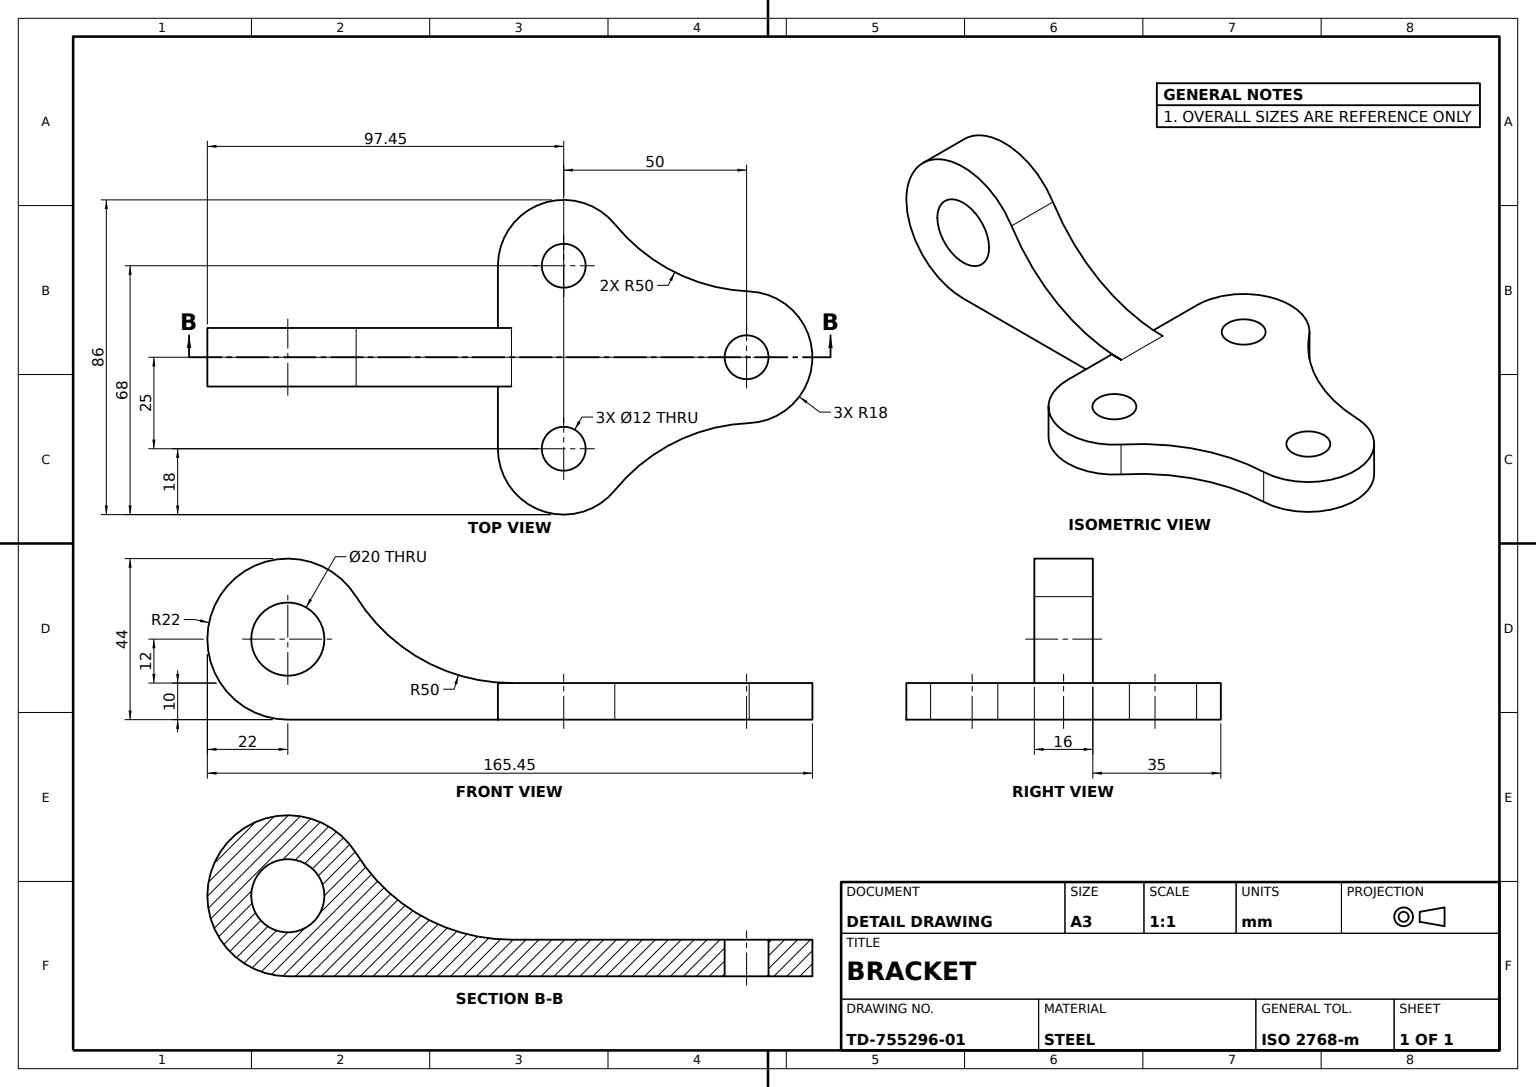
SolidWorks part; units mm, degrees
material "Plain Carbon Steel"
ref_plane "Front Plane" through (0, 0, 0) normal (0, 0, 1) x (1, 0, 0)
ref_plane "Top Plane" through (0, 0, 0) normal (0, 1, 0) x (1, 0, 0)
ref_plane "Right Plane" through (0, 0, 0) normal (1, 0, 0) x (0, 0, -1)
sketch "Arm Profile Sketch" plane through (0, 0, 0) normal (0, 0, 1) x (1, 0, 0)
  line L0 (-82.8947, 0) -> (86, 0) construction
  line L1 (0, 90.6316) -> (0, -108.8684) construction
  line L2 (0, 0) -> (0, 10)
  line L3 (0, 10) -> (86, 10)
  line L4 (86, 10) -> (86, 0)
  line L5 (86, 0) -> (0, 0)
  line L6 (-41, 0) -> (0, 0)
  circle A0 centre (-41, 22) radius 10
  arc A1 (-22.3136, 33.6111) -> (-41, 0) centre (-41, 22) ccw
  arc A2 (-22.3136, 33.6111) -> (20.1555, 10) centre (20.1555, 60) ccw
  dimension "D3" = 20
  dimension "D4" = 44
  dimension "D7" = 50
  dimension "D1" = 86
  dimension "D2" = 10
  dimension "D5" = 41
  dimension "D6" = 22
extrude "Arm Body" add sketch "Arm Profile Sketch" along normal mid plane 16 contours A2 A1 L6 L2 L3 A0
sketch "Mounting Flange Sketch" plane through (0, 10, 0) normal (0, 1, 0) x (1, 0, 0)
  line L0 (-16.3933, 0) -> (108.8818, 0) construction
  line L1 (20.1555, -8) -> (20.1555, 8) construction
  line L2 (16.4455, 25) -> (16.4455, -25)
  arc A0 (48.4016, 36.3679) -> (16.4455, 25) centre (34.4455, 25) ccw
  arc A1 (16.4455, -25) -> (48.4016, -36.3679) centre (34.4455, -25) ccw
  arc A2 (85.1663, -17.9856) -> (85.1663, 17.9856) centre (84.4455, 0) ccw
  circle A3 centre (84.4455, 0) radius 6
  circle A4 centre (34.4455, 25) radius 6
  circle A5 centre (34.4455, -25) radius 6
  arc A6 (48.4016, 36.3679) -> (85.1663, 17.9856) centre (87.1683, 67.9455) ccw
  arc A7 (48.4016, -36.3679) -> (85.1663, -17.9856) centre (87.1683, -67.9455) cw
  dimension "D5" = 12
  dimension "D6" = 36
  dimension "D7" = 50
  dimension "D1" = 14.29
  dimension "D2" = 14.29
  dimension "D3" = 50
  dimension "D4" = 50
  dimension "D8" = 68.7207
extrude "Mounting Flange" add sketch "Mounting Flange Sketch" against normal blind 10
sketch "Trim Cut Sketch" plane through (0, 10, 0) normal (0, 1, 0) x (1, 0, 0)
  line L0 (0, 0) -> (115.8988, 0) construction
  line L1 (34.4455, 25) -> (34.4455, -25)
  circle A0 centre (84.4455, 0) radius 6
  dimension "D1" = 50
extrude "Trim Cut" cut sketch "Trim Cut Sketch" against normal through all contours A0
